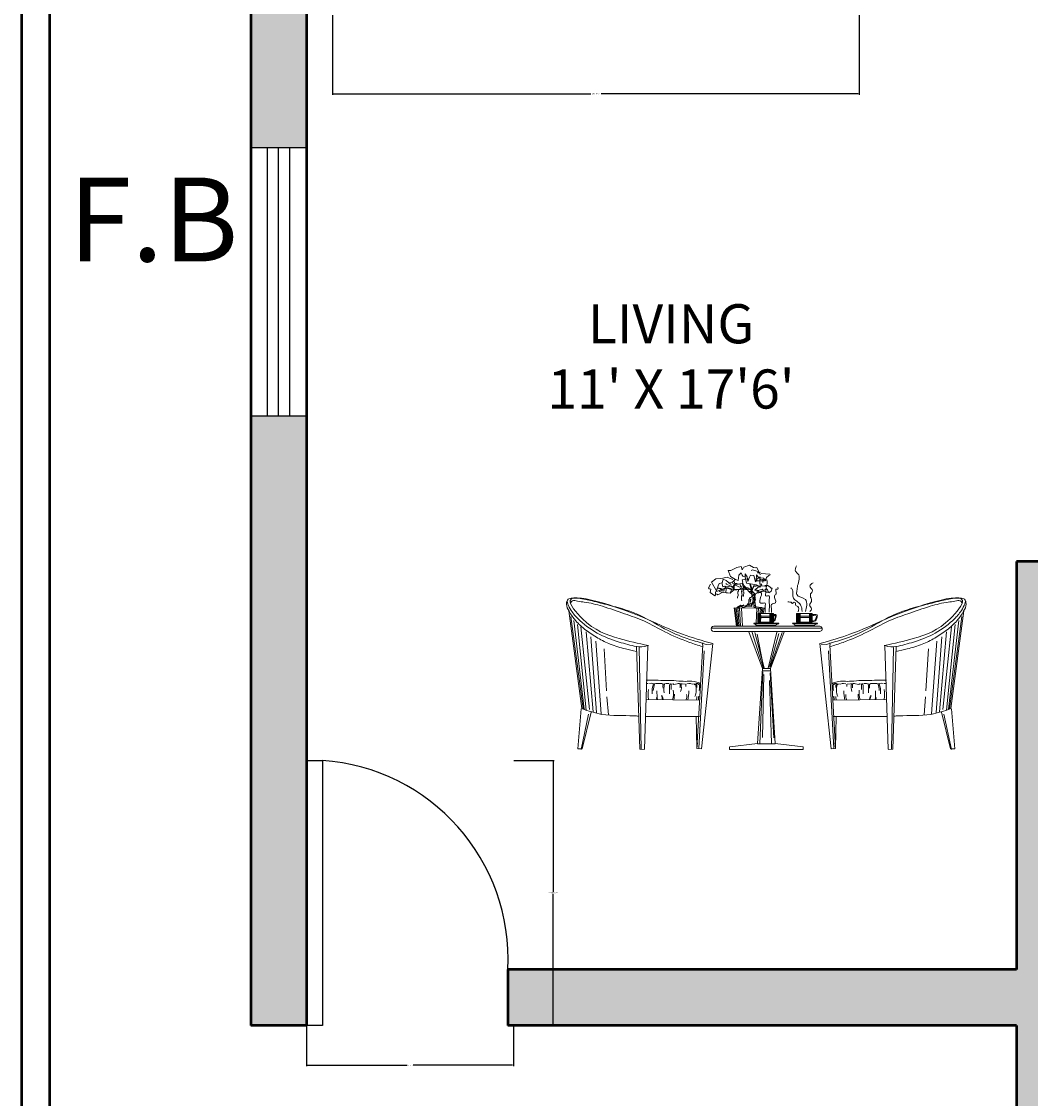
# Model space of a CAD drawing. Units: inches. Extents: x 1771 to 3025, y 319 to 889.
# Tile 26 of 35: x 2683 to 2863, y 521 to 714. Entities that reach past the tile are written whole.
import ezdxf

# ---------------------------------------------------------------- set-up
doc = ezdxf.new("R2010")
doc.units = ezdxf.units.IN
doc.header["$MEASUREMENT"] = 0
for name, color, linetype, lineweight in [('A-ANNO-DIMS', 2, 'Continuous', 18), ('A-AREA-IDEN', 241, 'Continuous', 25), ('A-DOOR', 4, 'Continuous', 25), ('A-FURN', 8, 'Continuous', 18), ('A-GLAZ', 40, 'Continuous', 25), ('A-WALL', 7, 'Continuous', 50), ('A-WALL-PATT', 254, 'Continuous', 13)]:
    doc.layers.add(name, color=color, linetype=linetype, lineweight=lineweight)
doc.styles.get("Standard").update_dxf_attribs({"font": 'arial.ttf'})
doc.dimstyles.get("Standard").update_dxf_attribs({"dimtxt": 0.18, "dimasz": 0.18, "dimexe": 0.18, "dimexo": 0.0625, "dimgap": 0.09, "dimtad": 0, "dimtih": 1, "dimtoh": 1, "dimdec": 4, "dimzin": 0, "dimdsep": 46, "dimtxsty": 'Standard', "dimcen": 0.09, "dimadec": 0, "dimazin": 0, "dimtfac": 1, "dimtdec": 4, "dimtofl": 0, "dimtmove": 0, "dimatfit": 3, "dimfxl": 1, "dimtolj": 1, "dimtzin": 0, "dimarcsym": 0})

# ---------------------------------------------------------------- blocks, each defined once
blk = doc.blocks.new('A$C7D4176DC')
for p, q in [((1010.5, 1037.1), (1041.4, 1048.3)), ((1041.4, 1048.3), (1064.8, 1036.1)), ((914, 980.9), (889.6, 974.3)), ((947.7, 967.8), (914, 980.9)), ((936.5, 1019.3), (919.6, 1018.3)), ((919.6, 1018.3), (933.7, 984.6)), ((933.7, 984.6), (961.8, 966.8)), ((969.3, 1036.1), (936.5, 1019.3)), ((994.5, 1040.8), (969.3, 1036.1)), ((976.7, 961.2), (980.5, 991.2)), ((980.5, 991.2), (994.5, 1005.2)), ((1000.2, 1022.1), (994.5, 1040.8)), ((994.5, 1005.2), (999.2, 992.1)), ((999.2, 992.1), (1006.7, 983.7)), ((1008.6, 1036.1), (1000.2, 1022.1)), ((1006.7, 983.7), (1022.6, 987.4)), ((1022.6, 987.4), (1015.2, 989.3)), ((1029.2, 982.8), (1017, 998.7)), ((1017, 998.7), (1017, 981.8)), ((1017, 981.8), (1024.5, 946.2)), ((1032, 956.5), (1029.2, 982.8)), ((1047.9, 992.1), (1042.3, 979.9)), ((1066.7, 989.3), (1047.9, 992.1)), ((1051.7, 1018.3), (1059.2, 1023)), ((1059.2, 1023), (1090.1, 1013.6)), ((1064.8, 1036.1), (1077, 1034.2)), ((1075.1, 953.7), (1066.7, 989.3)), ((1077, 1034.2), (1084.5, 1035.2)), ((1081.7, 994), (1079.8, 959.4)), ((1095.7, 976.2), (1081.7, 994)), ((1084.5, 1035.2), (1097.6, 1007.1)), ((1103.2, 982.8), (1084.5, 969.7)), ((1091, 1009.9), (1088.2, 1005.2)), ((1088.2, 1005.2), (1104.1, 1009)), ((1090.1, 1013.6), (1091, 1009.9)), ((1104.1, 1009), (1091, 1005.2)), ((1091, 1005.2), (1100.4, 1003.4)), ((1100.4, 1003.4), (1103.2, 993.1)), ((1100.4, 971.5), (1103.2, 982.8)), ((1108.2, 1001.8), (1157.5, 996.8)), ((1151, 989.3), (1137.9, 978.1)), ((1159.4, 994), (1151, 989.3)), ((1157.5, 996.8), (1159.4, 994)), ((820.3, 941.6), (808.1, 920)), ((808.1, 920), (811.9, 913.5)), ((850.3, 971.5), (825.9, 951.9)), ((825.9, 951.9), (853.1, 902.3)), ((879.3, 973.4), (850.3, 971.5)), ((853.1, 902.3), (863.4, 931.3)), ((863.4, 931.3), (869, 944.4)), ((869, 944.4), (886.8, 949.1)), ((889.6, 974.3), (879.3, 973.4)), ((890.6, 924.7), (884, 950)), ((886.8, 949.1), (892.4, 968.7)), ((900.9, 928.5), (890.6, 924.7)), ((892.4, 968.7), (908.4, 962.2)), ((922.4, 927.5), (900.9, 928.5)), ((903.7, 927.5), (902.7, 916.3)), ((905.6, 928.5), (903.7, 927.5)), ((904.6, 923.8), (905.6, 928.5)), ((904.6, 920), (904.6, 923.8)), ((919.6, 920), (904.6, 920)), ((908.4, 962.2), (934.6, 940.6)), ((909.3, 940.6), (908.4, 947.2)), ((917.7, 936), (909.3, 940.6)), ((928, 933.1), (917.7, 936)), ((939.3, 913.5), (919.6, 920)), ((932.7, 929.4), (922.4, 927.5)), ((927.4, 947.9), (955.2, 956.5)), ((942.1, 925.7), (928, 933.1)), ((941.1, 929.4), (932.7, 929.4)), ((934.6, 940.6), (938.3, 938.8)), ((951.5, 911.6), (941.1, 929.4)), ((950.5, 917.2), (942.1, 925.7)), ((946.8, 953.7), (945.8, 946.2)), ((945.8, 946.2), (971.1, 945.3)), ((958, 965.9), (946.8, 953.7)), ((955.2, 940.6), (946.8, 924.7)), ((946.8, 924.7), (951.5, 918.2)), ((959.9, 938.8), (951.5, 925.7)), ((951.5, 925.7), (954.3, 912.5)), ((954.3, 909.7), (955.2, 940.6)), ((955.2, 956.5), (961.8, 934.1)), ((986.1, 943.4), (960.8, 940.6)), ((961.8, 966.8), (976.7, 961.2)), ((961.8, 934.1), (984.2, 923.8)), ((967.4, 939.2), (999.2, 945.3)), ((984.2, 923.8), (995.5, 925.7)), ((989.9, 930.3), (986.1, 943.4)), ((989.5, 915.7), (998.5, 919.9)), ((995.5, 925.7), (989.9, 930.3)), ((998.5, 919.9), (1000.6, 912.2)), ((999.2, 965.9), (1016.1, 967.8)), ((1003, 952.8), (999.2, 965.9)), ((999.2, 945.3), (1003, 952.8)), ((1002, 948.1), (1001.1, 940.6)), ((1001.1, 940.6), (1006.7, 926.6)), ((1012.3, 931.3), (1002, 948.1)), ((1007.7, 920), (1005.8, 917.2)), ((1006.7, 926.6), (1011.4, 921.9)), ((1027.3, 916.3), (1007.7, 920)), ((1009.7, 920.6), (1011.8, 911.5)), ((1011.4, 921.9), (1025.5, 914.4)), ((1021.7, 921.9), (1012.3, 931.3)), ((1016.1, 967.8), (1017, 970.6)), ((1017, 970.6), (1037.6, 969.7)), ((1033, 919.1), (1021.7, 921.9)), ((1024.5, 946.2), (1082.6, 936)), ((1042.3, 979.9), (1032, 956.5)), ((1037.6, 969.7), (1033, 971.5)), ((1047.9, 941.6), (1043.3, 939.7)), ((1043.3, 939.7), (1048.9, 920)), ((1055.4, 914.4), (1047.9, 941.6)), ((1048.9, 920), (1049.8, 910.7)), ((1067.6, 934.1), (1054.5, 910.7)), ((1064.8, 923.8), (1061.1, 918.2)), ((1067.6, 929.4), (1064.8, 927.5)), ((1066.7, 926.6), (1064.8, 923.8)), ((1089.2, 931.3), (1066.7, 926.6)), ((1084.5, 932.2), (1067.6, 929.4)), ((1079.8, 959.4), (1075.1, 953.7)), ((1078.2, 913), (1100.1, 932)), ((1082.6, 936), (1096.7, 928.5)), ((1084.5, 969.7), (1084.5, 959.4)), ((1084.5, 959.4), (1127.6, 960.3)), ((1121, 975.3), (1095.7, 976.2)), ((1096.7, 928.5), (1101.3, 922.8)), ((1100.1, 932), (1097.2, 927.6)), ((1097.2, 927.6), (1117.7, 930.5)), ((1101.3, 940.6), (1100.4, 971.5)), ((1101.3, 922.8), (1111.6, 941.6)), ((1111.6, 941.6), (1101.3, 940.6)), ((1106, 966.8), (1104.1, 968.7)), ((1121, 969.7), (1106, 966.8)), ((1117.7, 930.5), (1139.6, 927.6)), ((1119.1, 963.1), (1121, 969.7)), ((1127.6, 960.3), (1119.1, 963.1)), ((1132.2, 960.3), (1121, 975.3)), ((1129.4, 933.4), (1145.5, 933.4)), ((1137.9, 978.1), (1132.2, 960.3)), ((1145.5, 933.4), (1160.1, 923.2)), ((1160.1, 923.2), (1166, 918.8)), ((811.9, 913.5), (821.2, 911.6)), ((821.2, 911.6), (817.5, 893.8)), ((817.5, 893.8), (843.7, 875.1)), ((843.7, 875.1), (847.5, 880.7)), ((847.5, 897.6), (877.4, 906)), ((847.5, 880.7), (847.5, 897.6)), ((862.1, 880.4), (853.9, 886.5)), ((860.6, 917.2), (858.7, 916.3)), ((863.4, 917.2), (860.6, 917.2)), ((878.4, 916.3), (861.5, 919.1)), ((886.7, 892.7), (862.1, 880.4)), ((876.5, 911.6), (863.4, 917.2)), ((870.3, 898.8), (868.3, 907)), ((895, 892.7), (870.3, 898.8)), ((879.3, 906.9), (876.5, 911.6)), ((877.4, 906), (884.9, 905.1)), ((883.1, 912.5), (878.4, 916.3)), ((894.3, 912.5), (879.3, 906.9)), ((910.2, 917.2), (883.1, 912.5)), ((884.9, 905.1), (889.6, 903.2)), ((889.6, 903.2), (895.2, 901.3)), ((902.7, 916.3), (894.3, 912.5)), ((931.9, 888.6), (895, 892.7)), ((895.2, 901.3), (899, 917.2)), ((909.3, 913.2), (907.3, 892.7)), ((917.5, 890.6), (909.3, 890.6)), ((939.3, 910.7), (910.2, 917.2)), ((931.9, 888.6), (917.5, 890.6)), ((940.1, 909.1), (931.9, 888.6)), ((950.4, 907), (931.9, 888.6)), ((985.2, 912.5), (939.3, 910.7)), ((1026.4, 913.5), (950.4, 907.4)), ((952.4, 910.7), (950.5, 917.2)), ((951.5, 918.2), (951.5, 911.6)), ((954.3, 912.5), (954.3, 909.7)), ((977.6, 875.3), (973.4, 867.6)), ((973.4, 867.6), (973.4, 860.6)), ((976.2, 896.9), (974.8, 892)), ((974.8, 892), (977.6, 877.4)), ((978.3, 903.2), (976.2, 896.9)), ((977.6, 912.2), (978.3, 903.2)), ((977.6, 877.4), (977.6, 875.3)), ((988.9, 914.4), (985.2, 912.5)), ((991.7, 916.3), (988.9, 914.4)), ((1005.8, 917.2), (991.7, 916.3)), ((998.5, 904.6), (995.7, 898.3)), ((995.7, 898.3), (999.9, 878.8)), ((997.1, 872.5), (996.4, 855.8)), ((999.9, 878.8), (997.1, 872.5)), ((1000.6, 912.2), (998.5, 904.6)), ((1006.9, 906), (1004.1, 898.3)), ((1004.1, 898.3), (1009, 894.8)), ((1008.3, 872.5), (1004.8, 871.8)), ((1011.8, 911.5), (1006.9, 906)), ((1006.9, 911.5), (1030.6, 908)), ((1009, 889.2), (1006.9, 877.4)), ((1006.9, 877.4), (1008.3, 872.5)), ((1009, 894.8), (1009, 889.2)), ((1025.5, 914.4), (1048.9, 908.8)), ((1030.6, 908), (1036.9, 901.1)), ((1046.7, 908.7), (1033, 919.1)), ((1036.9, 901.1), (1049.5, 899)), ((1039, 899), (1045.3, 891.3)), ((1049.5, 899), (1039, 899)), ((1044.6, 864.1), (1039.7, 853)), ((1050.9, 864.8), (1044.6, 864.1)), ((1045.3, 891.3), (1052.3, 886.4)), ((1048.9, 908.8), (1076, 881.7)), ((1049.8, 910.7), (1050.8, 902.3)), ((1050.8, 902.3), (1060.1, 872.3)), ((1058.2, 880.7), (1050.8, 894.8)), ((1055.8, 873.9), (1050.9, 864.8)), ((1052.3, 886.4), (1057.9, 876.7)), ((1054.5, 910.7), (1054.5, 898.5)), ((1054.5, 898.5), (1059.9, 896.9)), ((1056.4, 890.1), (1055.4, 914.4)), ((1056.4, 905.1), (1055.4, 895.7)), ((1055.4, 895.7), (1057.3, 892)), ((1057.9, 876.7), (1055.8, 873.9)), ((1061.1, 918.2), (1056.4, 905.1)), ((1064.4, 865.4), (1056.9, 822.4)), ((1060.1, 872.3), (1058.2, 880.7)), ((1069.5, 859.2), (1059.2, 870.4)), ((1065.7, 884.5), (1061.1, 875.1)), ((1061.1, 875.1), (1061.1, 857.3)), ((1064.8, 853.6), (1069.5, 859.2)), ((1074.2, 859.2), (1065.7, 884.5)), ((1070.4, 864.8), (1065.7, 823.6)), ((1070.4, 862.9), (1067.6, 890.1)), ((1076, 851.7), (1070.4, 864.8)), ((1074.2, 829.2), (1070.4, 862.9)), ((1076, 881.7), (1071.4, 876)), ((1071.4, 876), (1073.2, 863.9)), ((1072.3, 910), (1078.2, 913)), ((1091.3, 904.2), (1072.3, 910)), ((1073.2, 863.9), (1074.2, 859.2)), ((1076.7, 886.6), (1073.8, 883.7)), ((1097.2, 895.4), (1076.7, 886.6)), ((1098.6, 893.9), (1089.9, 904.2)), ((1113.3, 911.5), (1091.3, 904.2)), ((1113.3, 902.7), (1097.2, 895.4)), ((1113.3, 899.8), (1098.6, 893.9)), ((1122.1, 904.2), (1113.3, 911.5)), ((1127.9, 901.3), (1113.3, 899.8)), ((1138.2, 914.4), (1122.1, 904.2)), ((1138.2, 895.4), (1127.9, 901.3)), ((1144, 908.6), (1138.2, 914.4)), ((1151.3, 895.4), (1138.2, 895.4)), ((1151.3, 891), (1144, 908.6)), ((1166, 901.3), (1151.3, 891)), ((1166, 918.8), (1170.4, 917.3)), ((1170.4, 917.3), (1166, 901.3)), ((968.4, 700.9), (955.2, 806.2)), ((955.2, 806.2), (1126.5, 803.3)), ((959.3, 806.1), (972.5, 701.9)), ((965.6, 806.1), (976.7, 700.5)), ((991.6, 820.2), (969.9, 808.3)), ((975.3, 805.4), (983, 701.2)), ((979.4, 811.3), (977.9, 801.1)), ((991.8, 816.4), (978.6, 806.2)), ((985.8, 805.4), (990.6, 701.9)), ((1016.7, 816), (991.6, 820.2)), ((1003.5, 807.6), (991.8, 816.4)), ((996.2, 804.1), (1001.1, 701.9)), ((996.4, 855.8), (996.4, 850.9)), ((996.4, 850.9), (997.8, 845.3)), ((1009.4, 822.3), (1002, 816.4)), ((1002, 816.4), (1054.7, 813.5)), ((1013.7, 810.6), (1003.5, 807.6)), ((1041.6, 819.3), (1013.7, 810.6)), ((1060.6, 835.8), (1015.2, 815.4)), ((1022.3, 819.5), (1016.7, 816)), ((1024.4, 819.5), (1022.3, 819.5)), ((1026.5, 819.5), (1024.4, 819.5)), ((1029.9, 828.6), (1026.5, 819.5)), ((1032, 829.3), (1029.9, 828.6)), ((1033.4, 828.6), (1032, 829.3)), ((1036.9, 832), (1033.4, 828.6)), ((1037.6, 834.1), (1036.9, 832)), ((1044.5, 828.1), (1037.2, 822.3)), ((1037.2, 822.3), (1041.6, 819.3)), ((1039, 850.9), (1037.6, 836.2)), ((1037.6, 836.2), (1037.6, 834.1)), ((1039.7, 853), (1039, 850.9)), ((1048.9, 832.5), (1044.5, 828.1)), ((1048.1, 856.4), (1045.3, 850.2)), ((1045.3, 850.2), (1045.3, 839)), ((1045.3, 839), (1048.1, 841.1)), ((1048.1, 841.1), (1048.8, 853.7)), ((1048.8, 853.7), (1048.8, 857.1)), ((1057.7, 829.6), (1048.9, 832.5)), ((1049.8, 817.1), (1076, 851.7)), ((1051.7, 827.4), (1049.8, 817.1)), ((1054.7, 813.5), (1057.7, 829.6)), ((1061.1, 857.3), (1064.8, 853.6)), ((1065.7, 823.6), (1077, 814.3)), ((1066.4, 817.9), (1066.4, 812)), ((1066.4, 812), (1075.2, 806.2)), ((1075.2, 806.2), (1073.8, 812)), ((1073.8, 812), (1114.7, 807.6)), ((1077, 814.3), (1074.2, 829.2)), ((1098.2, 804.7), (1077.7, 804.7)), ((1083.8, 803.4), (1080.4, 718.8)), ((1093.6, 804.7), (1091.9, 774.3)), ((1114.7, 807.6), (1097.2, 801.8)), ((1104, 802), (1101.5, 774.3)), ((1110.9, 799.9), (1108, 774.3)), ((1117.9, 803.4), (1113.7, 774.3)), ((1125, 803.3), (1120, 774.3)), ((13.4, 788.5), (86.9, 232)), ((24.7, 755.7), (94.7, 231.2)), ((976.6, 787.5), (968.6, 786.7)), ((968.6, 786.7), (971.7, 756.8)), ((971.7, 756.8), (979.7, 757.6)), ((979.7, 757.6), (976.6, 787.5)), ((1088.8, 774.3), (1088.8, 724.7)), ((1179, 774.3), (1088.8, 774.3)), ((1100.8, 759), (1088.8, 759)), ((1100.8, 751.4), (1090.1, 751.4)), ((1090.9, 774.1), (1090.9, 725.1)), ((1093.9, 773.8), (1093.9, 725.1)), ((1098.4, 774.1), (1098.4, 724.9)), ((1100.8, 763.6), (1100.8, 747.6)), ((1107.3, 763.6), (1100.8, 763.6)), ((1100.8, 747.6), (1107.3, 747.6)), ((1101.3, 745), (1101.3, 740.5)), ((1107.3, 745), (1101.3, 745)), ((1101.3, 740.5), (1107.3, 740.5)), ((1104.1, 773.8), (1104.1, 763.6)), ((1104.1, 747.6), (1104.1, 745)), ((1104.1, 740.5), (1104.1, 724.7)), ((1107.3, 747.6), (1107.3, 763.6)), ((1179, 759), (1107.3, 759)), ((1179, 751.4), (1107.3, 751.4)), ((1107.3, 740.5), (1107.3, 745)), ((1158.2, 773.8), (1158.2, 725.1)), ((1164.1, 773.8), (1164.1, 724.9)), ((1168.6, 774.3), (1168.6, 725.4)), ((1172.9, 774.1), (1172.9, 767.4)), ((1172.9, 762.7), (1172.9, 734.9)), ((1175.9, 774.1), (1175.9, 767.3)), ((1175.9, 762.6), (1175.9, 734.6)), ((1178, 773.8), (1178, 767.2)), ((1178.3, 762.6), (1178.3, 734.8)), ((1179, 767.3), (1179, 774.3)), ((1179, 734.4), (1179, 762.7)), ((1309.2, 774.3), (1309.2, 724.7)), ((1399.4, 774.3), (1309.2, 774.3)), ((1319.1, 759), (1309.2, 759)), ((1319.1, 751.4), (1310.5, 751.4)), ((1311, 774.3), (1311, 725)), ((1313.8, 774.6), (1313.8, 724)), ((1318.3, 774.3), (1318.3, 725.2)), ((1319.1, 764.9), (1319.1, 742.2)), ((1323.5, 764.9), (1319.1, 764.9)), ((1319.1, 742.2), (1323.5, 742.2)), ((1319.8, 739.2), (1319.8, 735.6)), ((1322.7, 739.2), (1319.8, 739.2)), ((1322.7, 735.6), (1322.7, 739.2)), ((1323.5, 742.2), (1323.5, 764.9)), ((1399.4, 759), (1323.5, 759)), ((1399.4, 751.4), (1323.5, 751.4)), ((1324.3, 774.1), (1324.3, 725.5)), ((1331.2, 774.1), (1331.2, 725)), ((1383.9, 774.1), (1383.9, 725.2)), ((1389.2, 774.1), (1389.2, 724.8)), ((1393.7, 774.1), (1393.7, 724.5)), ((1396.6, 774.1), (1396.6, 724.8)), ((1398.3, 774.1), (1398.3, 724.8)), ((1399.4, 724.7), (1399.4, 774.3)), ((2250.4, 755.7), (2180.4, 231.2)), ((2261.7, 788.5), (2188.2, 232)), ((41.1, 733.1), (100.8, 229.1)), ((61.7, 710.4), (111.1, 223)), ((82.3, 698.1), (131.7, 227.1)), ((1452.4, 690.9), (826.8, 690.9)), ((1438.5, 700.9), (838.5, 700.9)), ((1107.4, 700.9), (968.4, 700.9)), ((1206.9, 718.8), (1068.5, 718.8)), ((1205.1, 715), (1070.7, 715)), ((1079.9, 707.4), (1079.6, 701.2)), ((1192.2, 706.1), (1080.1, 706.6)), ((1191.5, 704.8), (1081.7, 704.8)), ((1083.3, 700.5), (1083.3, 704.5)), ((1088.8, 724.7), (1179, 724.7)), ((1093.2, 718.3), (1093.2, 724.5)), ((1172.9, 732.2), (1172.9, 725.1)), ((1173.3, 725.1), (1173.3, 718.3)), ((1175.9, 731.8), (1175.9, 724.6)), ((1178.3, 731.3), (1178.3, 725.1)), ((1179, 724.7), (1179, 731.4)), ((1189, 704.5), (1189, 700.5)), ((1427.3, 718.8), (1288.9, 718.8)), ((1425.4, 715), (1291, 715)), ((1412.6, 706.1), (1300.5, 706.6)), ((1411.9, 704.8), (1302.1, 704.8)), ((1303.7, 700.5), (1303.7, 704.5)), ((1309.2, 724.7), (1399.4, 724.7)), ((1313.5, 718.3), (1313.5, 724.5)), ((1319.8, 735.6), (1322.7, 735.6)), ((1393.7, 725.1), (1393.7, 718.3)), ((1409.4, 704.5), (1409.4, 700.5)), ((2192.8, 698.1), (2143.4, 227.1)), ((2213.3, 710.4), (2163.9, 223)), ((2233.9, 733.1), (2174.2, 229.1)), ((111.1, 669.3), (152.3, 214.7)), ((137.9, 640.5), (170.8, 210.6)), ((166.7, 615.8), (197.6, 202.4)), ((1438.5, 670.9), (838.5, 670.9)), ((1037.2, 670.1), (1115.4, 459.8)), ((1054.9, 670.7), (1122.1, 460.1)), ((1073, 665.2), (1125.7, 463.7)), ((1085.8, 656.2), (1122.1, 471)), ((1198.4, 667), (1147.5, 461.9)), ((1209.3, 659.8), (1156.6, 467.4)), ((1227.5, 665.2), (1160.2, 467.4)), ((1239.7, 670.1), (1161.5, 459.8)), ((2108.4, 615.8), (2077.5, 202.4)), ((2137.2, 640.5), (2104.3, 210.6)), ((2163.9, 669.3), (2122.8, 214.7)), ((214, 572.6), (228.4, 334)), ((398.7, 587.3), (417.4, 0.9)), ((413.7, 579.8), (424.7, 0.9)), ((462.3, 591), (443.8, 0.9)), ((776.4, 594.8), (742.7, 4.4)), ((783.9, 560.6), (752.8, 5.4)), ((795.6, 597.2), (767.4, 606)), ((832.5, 602.2), (768.9, 2.8)), ((772.6, 598.5), (776.4, 598.5)), ((825, 598.5), (795.6, 597.2)), ((1442.6, 602.2), (1506.2, 2.8)), ((1450.1, 598.5), (1479.4, 597.2)), ((1479.4, 597.2), (1507.7, 606)), ((1491.2, 560.6), (1522.3, 5.4)), ((1502.4, 598.5), (1498.7, 598.5)), ((1498.7, 594.8), (1532.3, 4.4)), ((1812.8, 591), (1831.2, 0.9)), ((1861.4, 579.8), (1850.3, 0.9)), ((1876.4, 587.3), (1857.7, 0.9)), ((2061, 572.6), (2046.6, 334)), ((1115.4, 459.8), (1088.3, 33.1)), ((1118.5, 442), (1100.3, 33.5)), ((1163.9, 447.4), (1114.8, 447.4)), ((1161.5, 459.8), (1115.4, 459.8)), ((1160.2, 436.5), (1180.2, 66.2)), ((1161.5, 459.8), (1188.6, 33.1)), ((465.7, 375.8), (456.5, 375.8)), ((484.1, 377.3), (471.9, 374.3)), ((499.5, 372.7), (484.1, 377.3)), ((508.7, 374.3), (499.5, 372.7)), ((513.3, 375.8), (508.7, 374.3)), ((525.5, 375.8), (513.3, 375.8)), ((531.7, 374.3), (525.5, 375.8)), ((543.9, 374.3), (531.7, 374.3)), ((547, 371.2), (543.9, 374.3)), ((567, 375.8), (547, 371.2)), ((582.3, 374.3), (567, 375.8)), ((593, 371.2), (590, 374.3)), ((606.8, 372.7), (593, 371.2)), ((611.4, 369.7), (606.8, 372.7)), ((629.8, 372.7), (611.4, 369.7)), ((636, 374.3), (629.8, 372.7)), ((643.6, 375.8), (636, 374.3)), ((648.2, 372.7), (643.6, 375.8)), ((659, 372.7), (648.2, 372.7)), ((677.4, 371.2), (659, 372.7)), ((678.9, 371.2), (678.9, 359)), ((697.3, 374.3), (685.1, 372.7)), ((706.5, 374.3), (697.3, 374.3)), ((715.7, 371.2), (706.5, 374.3)), ((729.5, 372.7), (715.7, 371.2)), ((740.3, 374.3), (729.5, 368.2)), ((729.5, 368.2), (729.5, 372.7)), ((747.9, 374.3), (740.3, 374.3)), ((751, 369.7), (747.9, 374.3)), ((760.2, 374.3), (751, 369.7)), ((1123.9, 427.4), (1116.6, 68)), ((1154.8, 393), (1167.5, 35.4)), ((1514.9, 374.3), (1524.1, 369.7)), ((1524.1, 369.7), (1527.1, 374.3)), ((1527.1, 374.3), (1534.8, 374.3)), ((1534.8, 374.3), (1545.5, 368.2)), ((1545.5, 372.7), (1559.3, 371.2)), ((1545.5, 368.2), (1545.5, 372.7)), ((1559.3, 371.2), (1568.5, 374.3)), ((1568.5, 374.3), (1577.7, 374.3)), ((1577.7, 374.3), (1590, 372.7)), ((1596.2, 371.2), (1596.2, 359)), ((1597.7, 371.2), (1616.1, 372.7)), ((1616.1, 372.7), (1626.8, 372.7)), ((1626.8, 372.7), (1631.4, 375.8)), ((1631.4, 375.8), (1639.1, 374.3)), ((1639.1, 374.3), (1645.2, 372.7)), ((1645.2, 372.7), (1663.6, 369.7)), ((1663.6, 369.7), (1668.2, 372.7)), ((1668.2, 372.7), (1682, 371.2)), ((1682, 371.2), (1685.1, 374.3)), ((1692.8, 374.3), (1708.1, 375.8)), ((1708.1, 375.8), (1728.1, 371.2)), ((1728.1, 371.2), (1731.1, 374.3)), ((1731.1, 374.3), (1743.4, 374.3)), ((1743.4, 374.3), (1749.5, 375.8)), ((1749.5, 375.8), (1761.8, 375.8)), ((1761.8, 375.8), (1766.4, 374.3)), ((1766.4, 374.3), (1775.6, 372.7)), ((1775.6, 372.7), (1790.9, 377.3)), ((1790.9, 377.3), (1803.2, 374.3)), ((1809.3, 375.8), (1818.5, 375.8)), ((230.5, 299.1), (238.7, 196.2)), ((756.8, 280.8), (451.1, 284.6)), ((1518.3, 280.8), (1824, 284.6)), ((2044.6, 299.1), (2036.3, 196.2)), ((84, 230.1), (64.2, 2.8)), ((126, 200.5), (84, 0.3)), ((140.9, 212.8), (88.9, 2.8)), ((447.3, 187.5), (757.7, 187.5)), ((739, 187.5), (742.7, 4.4)), ((1827.8, 187.5), (1517.4, 187.5)), ((1536.1, 187.5), (1532.3, 4.4)), ((2134.2, 212.8), (2186.2, 2.8)), ((2149.1, 200.5), (2191.1, 0.3)), ((2191.1, 230.1), (2210.9, 2.8)), ((64.2, 2.8), (88.9, 2.8)), ((417.4, 0.9), (443.8, 0)), ((742.7, 4.4), (746.5, 38)), ((742.7, 4.4), (768.9, 2.8)), ((927.1, 15), (927.1, 0)), ((1088.3, 33.1), (929, 15)), ((1187.5, 31.7), (1087.6, 31.7)), ((1188.6, 33.1), (1348, 15)), ((1348, 15), (1348, 0)), ((1532.3, 4.4), (1506.2, 2.8)), ((1532.3, 4.4), (1528.6, 38)), ((1857.7, 0.9), (1831.3, 0)), ((2210.9, 2.8), (2186.2, 2.8)), ((1348, 0), (927.1, 0))]:
    blk.add_line(p, q)
for centre, radius, start, end in [((838.2, 685.9), 15, 89.02539, 270.97461), ((1069.4, 716.9), 2.21, 114.75071, 294.8305), ((1059.6, 691.4), 25.9, 31.12717, 65.45392), ((1208.6, 696.5), 19, 99.79621, 154.31096), ((1206.2, 716.7), 1.95, 244.55032, 96.50843), ((1289.8, 716.9), 2.21, 114.75071, 294.8305), ((1280, 691.4), 25.9, 31.12717, 65.45392), ((1429, 696.5), 19, 99.79621, 154.31096), ((1426.6, 716.7), 1.95, 244.55032, 96.50843), ((1440.2, 685.9), 15.1, 263.50595, 96.49405), ((421.9, 675.7), 92.7, 253.90068, 295.36386), ((1853.1, 675.7), 92.7, 244.63614, 286.09932), ((631.7, 325.3), 145, 160.46362, 183.26427), ((661.3, 321.8), 167.8, 162.1481, 175.52768), ((592, 359.5), 42.9, 161.29008, 193.50095), ((755.4, 341.1), 200.6, 170.95256, 185.34949), ((841.5, 337.8), 255.8, 172.03905, 184.65389), ((943.9, 345.9), 348.8, 175.42446, 180.75439), ((590.6, 356.2), 56.7, 354.25823, 16.89433), ((579.3, 354.7), 74.8, 340.32989, 13.94105), ((619.9, 341.7), 118.4, 339.52102, 14.35705), ((693.6, 357.6), 48.4, 353.58471, 16.22063), ((689.2, 351.2), 68.2, 347.09902, 16.48344), ((1585.8, 351.2), 68.2, 163.51656, 192.90098), ((1581.5, 357.6), 48.4, 163.77937, 186.41529), ((1655.1, 341.7), 118.4, 165.64295, 200.47898), ((1695.8, 354.7), 74.8, 166.05895, 199.67011), ((1684.4, 356.2), 56.7, 163.10567, 185.74177), ((1331.2, 345.9), 348.8, 359.24561, 4.57554), ((1433.6, 337.8), 255.8, 355.34611, 7.96095), ((1519.7, 341.1), 200.6, 354.65051, 9.04744), ((1683.1, 359.5), 42.9, 346.49905, 18.70992), ((1613.7, 321.8), 167.8, 4.47232, 17.8519), ((1643.3, 325.3), 145, 356.73573, 19.53638), ((665.2, 310.8), 200.4, 171.53233, 187.34342), ((746.2, 323.3), 231.2, 177.65923, 189.89094), ((596.6, 305.3), 53.4, 177.23164, 203.39317), ((484.6, 319.5), 124.8, 342.71731, 8.30681), ((204.5, 341.5), 411.6, 351.83053, 356.14259), ((645.6, 301.5), 39.5, 333.88539, 14.90767), ((494.8, 326.9), 201, 346.57929, 1.64099), ((1780.3, 326.9), 201, 178.35901, 193.42071), ((1629.4, 301.5), 39.5, 165.09233, 206.11461), ((2070.6, 341.5), 411.6, 183.85741, 188.16947), ((1790.4, 319.5), 124.8, 171.69319, 197.28269), ((1678.5, 305.3), 53.4, 336.60683, 2.76836), ((1528.9, 323.3), 231.2, 350.10906, 2.34077), ((1609.9, 310.8), 200.4, 352.65658, 8.46767), ((522.1, 292), 10.6, 155.04372, 216.38582), ((-475.8, 101.1), 1042.4, 10.14258, 11.10952), ((682.4, 301.4), 59.8, 341.0378, 359.49279), ((616.9, 303.9), 135.6, 349.74606, 359.61704), ((1658.2, 303.9), 135.6, 180.38296, 190.25394), ((1592.7, 301.4), 59.8, 180.50721, 198.9622), ((2750.9, 101.1), 1042.4, 168.89048, 169.85742), ((1753, 292), 10.6, 323.61418, 24.95628)]:
    blk.add_arc(centre, radius, start, end)
for points, knots in [([(1361.4, 785.9), (1364, 797.1), (1369.1, 819), (1366.1, 867.4), (1305.9, 865.7), (1312.3, 906.5), (1315.7, 942.7), (1336.1, 991.6), (1296, 1015.4), (1304.6, 1034), (1310, 1045.7)], [0, 0, 0, 0, 35.255511, 69.327341, 124.802742, 145.944632, 176.486081, 244.459642, 263.687549, 295.971636, 295.971636, 295.971636, 295.971636]), ([(1154.2, 782.2), (1154.8, 800.5), (1155.7, 825.5), (1152.5, 852.8), (1161, 880.4), (1126, 866.1), (1137.2, 896.5), (1131.8, 923.4), (1156.8, 968.1), (1113.4, 971.1), (1116.9, 957), (1118.7, 949.8)], [0, 0, 0, 0, 53.324624, 72.369114, 91.413604, 110.471764, 134.594802, 149.830446, 204.42477, 220.941926, 238.716972, 238.716972, 238.716972, 238.716972]), ([(1166.9, 779.6), (1167.6, 787.2), (1168.9, 801.7), (1159.5, 831.3), (1208.7, 829.6), (1171.7, 871.4), (1202, 885.9), (1182.6, 918), (1207, 909.8), (1204.8, 918.7), (1203.8, 923.1)], [0, 0, 0, 0, 24.123038, 45.706674, 71.213394, 110.655389, 125.899008, 152.561192, 162.725628, 172.882723, 172.882723, 172.882723, 172.882723]), ([(1341.7, 785.9), (1340.2, 798.9), (1337.5, 822.1), (1313, 843.2), (1292.5, 855.8), (1286.2, 880.3), (1292.2, 903.3), (1280.3, 916.5), (1276.7, 920.3)], [0, 0, 0, 0, 37.360481, 67.270583, 93.998428, 104.993238, 141.362472, 156.467713, 156.467713, 156.467713, 156.467713]), ([(1385.6, 784.4), (1390.4, 789.9), (1401.4, 802.3), (1375.2, 822.1), (1401.7, 842.3), (1389.4, 864.6), (1386.5, 887), (1411.5, 904.8), (1373.5, 930.7), (1394.6, 942.4), (1403.7, 947.5)], [0, 0, 0, 0, 18.925439, 42.566292, 64.867201, 90.936936, 109.058775, 128.752565, 161.181972, 185.77482, 185.77482, 185.77482, 185.77482]), ([(398, 584.9), (364.8, 593.1), (288.2, 612.1), (173, 656.7), (78.3, 727.2), (27.8, 785.3), (-11.1, 856.8), (24.4, 860.7), (34.5, 861.8)], [0, 0, 0, 0, 102.450812, 236.341037, 372.740804, 434.264952, 500.538568, 526.867635, 526.867635, 526.867635, 526.867635]), ([(832.5, 602.2), (773.3, 619.4), (552.4, 683.6), (381.9, 796.6), (-38, 894.8), (125.3, 689.4), (274.3, 633.7), (409.7, 603.5), (466, 591)], [0, 0, 0, 0, 179.241333, 669.878405, 853.517726, 978.360591, 1217.111989, 1387.04363, 1387.04363, 1387.04363, 1387.04363]), ([(778, 604.3), (747.1, 612.4), (671.2, 632.3), (544.7, 691), (406.7, 777.8), (262.4, 816.3), (152.4, 843.8), (83.7, 860.5), (45.9, 861.5), (34.5, 861.8)], [0, 0, 0, 0, 95.639299, 234.867324, 416.660896, 581.537135, 678.863317, 758.06805, 792.133261, 792.133261, 792.133261, 792.133261]), ([(1131.4, 779.6), (1130.3, 791.6), (1128.8, 807.5), (1135.2, 839.3), (1091.9, 821.5), (1105.3, 863.2), (1115.5, 900.9), (1079.7, 883.7), (1089.8, 909.5), (1078.6, 906.7), (1072.9, 905.3)], [0, 0, 0, 0, 39.358681, 52.054923, 76.195091, 115.553772, 137.137409, 158.736993, 171.43349, 184.13893, 184.13893, 184.13893, 184.13893]), ([(1442.6, 602.2), (1501.7, 619.4), (1722.7, 683.6), (1893.2, 796.6), (2313.1, 894.8), (2149.7, 689.4), (2000.7, 633.7), (1865.4, 603.5), (1809.1, 591)], [0, 0, 0, 0, 179.241333, 669.878405, 853.517726, 978.360591, 1217.111989, 1387.04363, 1387.04363, 1387.04363, 1387.04363]), ([(1497.1, 604.3), (1528, 612.4), (1603.8, 632.3), (1730.4, 691), (1868.3, 777.8), (2012.7, 816.3), (2122.7, 843.8), (2191.4, 860.5), (2229.2, 861.5), (2240.6, 861.8)], [0, 0, 0, 0, 95.639299, 234.867324, 416.660896, 581.537135, 678.863317, 758.06805, 792.133261, 792.133261, 792.133261, 792.133261]), ([(1877.1, 584.9), (1910.3, 593.1), (1986.9, 612.1), (2102.1, 656.7), (2196.8, 727.2), (2247.3, 785.3), (2286.2, 856.8), (2250.7, 860.7), (2240.6, 861.8)], [0, 0, 0, 0, 102.450812, 236.341037, 372.740804, 434.264952, 500.538568, 526.867635, 526.867635, 526.867635, 526.867635]), ([(397.9, 557.5), (377.2, 562.2), (327.1, 573.6), (252, 594.7), (177.4, 633.5), (110.3, 676.9), (52.9, 727.5), (17.7, 778.4), (-3, 818.5), (1.2, 838.8), (2.4, 844.5)], [0, 0, 0, 0, 63.757158, 154.207673, 233.111021, 314.773872, 393.990027, 459.45949, 503.309158, 520.507412, 520.507412, 520.507412, 520.507412]), ([(774.4, 584.9), (749.6, 592.8), (676.5, 616.3), (565.4, 663.8), (449, 732.3), (326.3, 773), (214.5, 813.5), (122.5, 837.9), (67.5, 840.8), (36.8, 851.9), (27.3, 839.8), (24.3, 836)], [0, 0, 0, 0, 78.234212, 230.212389, 361.399227, 482.184421, 615.817971, 721.353317, 759.79292, 789.08251, 802.845503, 802.845503, 802.845503, 802.845503]), ([(1319.1, 782.9), (1321.9, 795.4), (1325.6, 812.1), (1309.5, 816.4), (1302.3, 822.2), (1305.8, 830.8), (1295.5, 845.6), (1286, 822.9), (1281.2, 839.2), (1270.5, 838.4), (1264.1, 839.6), (1260.1, 840.3)], [0, 0, 0, 0, 30.24085, 40.376736, 46.786017, 54.336911, 66.135106, 80.063877, 89.736225, 97.441532, 109.625491, 109.625491, 109.625491, 109.625491]), ([(1500.6, 584.9), (1525.5, 592.8), (1598.5, 616.3), (1709.7, 663.8), (1826.1, 732.3), (1948.7, 773), (2060.6, 813.5), (2152.5, 837.9), (2207.6, 840.8), (2238.3, 851.9), (2247.7, 839.8), (2250.7, 836)], [0, 0, 0, 0, 78.234212, 230.212389, 361.399227, 482.184421, 615.817971, 721.353317, 759.79292, 789.08251, 802.845503, 802.845503, 802.845503, 802.845503]), ([(1877.1, 557.5), (1897.9, 562.2), (1947.9, 573.6), (2023.1, 594.7), (2097.7, 633.5), (2164.7, 676.9), (2222.2, 727.5), (2257.3, 778.4), (2278.1, 818.5), (2273.8, 838.8), (2272.7, 844.5)], [0, 0, 0, 0, 63.757158, 154.207673, 233.111021, 314.773872, 393.990027, 459.45949, 503.309158, 520.507412, 520.507412, 520.507412, 520.507412]), ([(1169.5, 767.6), (1169.1, 766.9), (1168.6, 765.8), (1168.5, 764.1), (1168.9, 763.4), (1169.1, 763)], [0, 0, 0, 0, 2.454471, 3.694729, 4.863756, 4.863756, 4.863756, 4.863756]), ([(1169.1, 763), (1172.8, 762.7), (1177.7, 762.3), (1183.6, 763.4), (1189.9, 762.9), (1187.4, 754.3), (1187.2, 747.1), (1184.4, 741.1), (1183.6, 734.2), (1179.1, 734.3), (1176.3, 734.5), (1173.7, 734.9), (1171.6, 734.9), (1169.1, 736.3), (1168.8, 734.4), (1168.7, 733.5), (1168.7, 732.9), (1169, 732.2), (1169.6, 732.2), (1169.9, 732.3)], [0, 0, 0, 0, 11.017731, 14.368752, 18.607743, 26.502791, 33.640107, 41.65747, 47.330925, 50.070533, 53.653147, 56.161165, 57.765785, 60.50412, 61.601302, 62.440841, 63.254964, 63.604793, 64.589255, 64.589255, 64.589255, 64.589255]), ([(1169.5, 767.6), (1173.2, 767.4), (1179.9, 766.9), (1197.8, 769.9), (1190.9, 747.3), (1187.7, 728.5), (1175.3, 732.4), (1169.7, 732.3), (1169.1, 732.2)], [0, 0, 0, 0, 11.640419, 20.980802, 45.0396, 57.043585, 71.929427, 73.92866, 73.92866, 73.92866, 73.92866]), ([(1180.5, 766.4), (1182.7, 766.7), (1186, 767.2), (1193.4, 764.4), (1189.7, 753.8), (1188.7, 747.3), (1188.2, 744.3)], [0, 0, 0, 0, 6.446326, 10.075492, 21.292554, 31.027811, 31.027811, 31.027811, 31.027811]), ([(1399.4, 767.3), (1402.9, 767.5), (1411.4, 768.1), (1432.6, 770.2), (1424.9, 746.9), (1419.3, 731), (1409, 728.9), (1399.9, 726.6), (1399.4, 728.7), (1399.4, 728.8)], [0, 0, 0, 0, 11.082717, 27.168464, 47.8303, 63.341794, 75.5235, 81.952599, 82.221535, 82.221535, 82.221535, 82.221535]), ([(1399.4, 760.8), (1402.3, 761.2), (1409.4, 762.1), (1423.2, 766.3), (1423.3, 753.9), (1420.3, 746.4), (1417.8, 735.7), (1409.3, 733.5), (1403.3, 729.7), (1400.4, 731.6), (1399.4, 732.3)], [0, 0, 0, 0, 9.652474, 22.996839, 29.518582, 40.146055, 49.702279, 58.739504, 65.130432, 68.539734, 68.539734, 68.539734, 68.539734]), ([(763.3, 374.3), (771.1, 374), (721.2, 391.5), (701, 387.4), (647.2, 387.1), (600.7, 394.2), (547.4, 391.8), (499.5, 394.7), (467.3, 394.3), (453.5, 394.2)], [0, 0, 0, 0, 23.359127, 69.600901, 112.546095, 167.952511, 215.499051, 270.735631, 312.147322, 312.147322, 312.147322, 312.147322]), ([(1511.8, 374.3), (1504, 374), (1553.9, 391.5), (1574.1, 387.4), (1627.8, 387.1), (1674.4, 394.2), (1727.7, 391.8), (1775.6, 394.7), (1807.8, 394.3), (1821.6, 394.2)], [0, 0, 0, 0, 23.359127, 69.600901, 112.546095, 167.952511, 215.499051, 270.735631, 312.147322, 312.147322, 312.147322, 312.147322]), ([(86.9, 232), (124.5, 219.1), (220.3, 186.2), (332, 194.5), (402.2, 190.3), (411.4, 189.7)], [0, 0, 0, 0, 118.259021, 301.591906, 329.266035, 329.266035, 329.266035, 329.266035]), ([(2188.2, 232), (2150.6, 219.1), (2054.8, 186.2), (1943.1, 194.5), (1872.9, 190.3), (1863.7, 189.7)], [0, 0, 0, 0, 118.259021, 301.591906, 329.266035, 329.266035, 329.266035, 329.266035])]:
    blk.add_open_spline(points, degree=3, knots=knots)
blk = doc.blocks.new('DOOR-36A')
blk.add_lwpolyline([(0, 47.37), (2.84, 47.37), (2.84, 0), (0, 0)], close=True)
blk.add_arc((0.47, 11.87), 35.58, 356.991, 86.1899)
blk = doc.blocks.new('WIN-48')
for p, q in [((0, 0), (0, 10)), ((48, 0), (48, 10)), ((0, 7), (48, 7)), ((0, 5), (48, 5)), ((0, 3), (48, 3))]:
    blk.add_line(p, q)
blk = doc.blocks.new('*D32')
at = {"layer": 'A-ANNO-DIMS', "color": 0, "lineweight": -2, "transparency": 16777216}
for p, q in [((2770.77, 581.85), (2777.99, 581.85)), ((2777.81, 581.67), (2777.81, 558.35)), ((2777.81, 534.66), (2777.81, 557.98)), ((2770.77, 534.48), (2777.99, 534.48))]:
    blk.add_line(p, q, dxfattribs=at)
at = {"layer": 'A-ANNO-DIMS', "color": 0, "transparency": 16777216}
for points in [[(2777.78, 581.67), (2777.84, 581.67), (2777.81, 581.85)], [(2777.78, 534.66), (2777.84, 534.66), (2777.81, 534.48)]]:
    blk.add_solid(points, dxfattribs=at)
at = {"layer": 'Defpoints', "color": 0, "transparency": 16777216}
for p in [(2770.71, 581.85), (2777.81, 581.85), (2770.71, 534.48)]:
    blk.add_point(p, dxfattribs=at)
at = {"layer": 'A-ANNO-DIMS', "color": 0, "transparency": 16777216, "insert": (2777.81, 558.17), "char_height": 0.18, "attachment_point": 5}
blk.add_mtext('\\A1;DOOR D3 47 TYP.', dxfattribs=at)
blk = doc.blocks.new('*D33')
at = {"layer": 'A-ANNO-DIMS', "color": 0, "lineweight": -2, "transparency": 16777216}
for p, q in [((2733.68, 534.42), (2733.68, 527.2)), ((2770.71, 534.42), (2770.71, 527.2)), ((2733.86, 527.38), (2751.67, 527.38)), ((2770.53, 527.38), (2752.72, 527.38))]:
    blk.add_line(p, q, dxfattribs=at)
at = {"layer": 'A-ANNO-DIMS', "color": 0, "transparency": 16777216}
for points in [[(2733.86, 527.41), (2733.86, 527.35), (2733.68, 527.38)], [(2770.53, 527.41), (2770.53, 527.35), (2770.71, 527.38)]]:
    blk.add_solid(points, dxfattribs=at)
at = {"layer": 'Defpoints', "color": 0, "transparency": 16777216}
for p in [(2733.68, 534.48), (2770.71, 534.48), (2770.71, 527.38)]:
    blk.add_point(p, dxfattribs=at)
at = {"layer": 'A-ANNO-DIMS', "color": 0, "transparency": 16777216, "insert": (2752.2, 527.38), "char_height": 0.18, "attachment_point": 5}
blk.add_mtext('\\A1;37 TYP.', dxfattribs=at)
blk = doc.blocks.new('*D46')
at = {"layer": 'A-ANNO-DIMS', "color": 0, "lineweight": -2, "transparency": 16777216}
for p, q in [((2738.34, 715.17), (2738.34, 700.92)), ((2832.56, 715.17), (2832.56, 700.92)), ((2738.52, 701.1), (2784.55, 701.1)), ((2832.38, 701.1), (2786.36, 701.1))]:
    blk.add_line(p, q, dxfattribs=at)
at = {"layer": 'A-ANNO-DIMS', "color": 0, "transparency": 16777216}
for points in [[(2738.52, 701.13), (2738.52, 701.07), (2738.34, 701.1)], [(2832.38, 701.13), (2832.38, 701.07), (2832.56, 701.1)]]:
    blk.add_solid(points, dxfattribs=at)
at = {"layer": 'Defpoints', "color": 0, "transparency": 16777216}
for p in [(2738.34, 715.24), (2832.56, 715.24), (2832.56, 701.1)]:
    blk.add_point(p, dxfattribs=at)
at = {"layer": 'A-ANNO-DIMS', "color": 0, "transparency": 16777216, "insert": (2785.45, 701.1), "char_height": 0.18, "attachment_point": 5}
blk.add_mtext('\\A1;SOFA 94 TYP.', dxfattribs=at)

msp = doc.modelspace()

# ---------------------------------------------------------------- hatches: boundary and pattern name
at = {"layer": 'A-WALL-PATT'}
h = msp.add_hatch(color=256, dxfattribs=at)
h.dxf.hatch_style = 1
h.paths.add_polyline_path([(2870.68, 879.48), (2892.73, 879.48), (2892.73, 889.48), (2842.68, 889.48), (2842.68, 879.48), (2865.68, 879.48), (2865.68, 831.48), (2870.68, 831.48)])
h.paths.add_polyline_path([(2983.64, 889.48), (2940.73, 889.48), (2940.73, 879.48), (2961.68, 879.48), (2961.68, 795.48), (2865.68, 795.48), (2865.68, 759.48), (2865.68, 665.48), (2870.68, 665.48), (2870.68, 712.85), (2870.68, 790.48), (2978.68, 790.48), (2978.68, 795.48), (2966.68, 795.48), (2966.68, 879.48), (2983.64, 879.48)])
h.paths.add_polyline_path([(3024.68, 889.48), (3001.64, 889.48), (3001.64, 879.48), (3014.68, 879.48), (3014.68, 790.48), (3014.68, 769.46), (3024.68, 769.46)])
h.paths.add_polyline_path([(3024.68, 721.46), (3014.68, 721.46), (3014.68, 670.48), (2906.68, 670.48), (2906.68, 665.48), (2925.68, 665.48), (2925.68, 653.48), (2930.68, 653.48), (2930.68, 665.48), (3014.68, 665.48), (3014.68, 650.02), (3024.68, 650.02)])
h.paths.add_polyline_path([(3024.68, 632.02), (3014.68, 632.02), (3014.68, 617.48), (2925.68, 617.48), (2906.68, 617.48), (2906.68, 612.48), (3014.68, 612.48), (3014.68, 581.96), (3024.68, 581.96)])
h.paths.add_polyline_path([(3024.68, 533.96), (3014.68, 533.96), (3014.68, 480.48), (2870.68, 480.48), (2870.68, 617.48), (2860.68, 617.48), (2860.68, 544.48), (2769.68, 544.48), (2769.68, 534.48), (2860.68, 534.48), (2860.68, 470.48), (3014.68, 470.48), (3014.68, 453.61), (3024.68, 453.61)])
h.paths.add_polyline_path([(3024.68, 405.61), (3014.68, 405.61), (3014.68, 394.48), (2860.68, 394.48), (2860.68, 384.48), (3024.68, 384.48)])
h.paths.add_polyline_path([(2733.68, 643.43), (2723.68, 643.43), (2723.68, 534.48), (2733.68, 534.48)])
h.paths.add_polyline_path([(2733.68, 754.48), (2829.68, 754.48), (2829.68, 759.48), (2733.68, 759.48), (2733.68, 843.44, -0.008336), (2732.38, 843.48), (2723.68, 843.48), (2723.68, 691.43), (2733.68, 691.43)])
h.paths.add_polyline_path([(2794.68, 889.48), (2723.68, 889.48), (2723.68, 879.48), (2794.68, 879.48)])

# ---------------------------------------------------------------- linework, layer by layer
at = {"layer": 'A-WALL'}
for p, q in [((2682.68, 889.48), (2682.68, 534.48)), ((2687.68, 879.48), (2687.68, 534.48)), ((2723.68, 843.48), (2723.68, 534.48)), ((2733.68, 754.48), (2733.68, 534.48)), ((2870.68, 617.48), (2860.68, 617.48)), ((2860.68, 617.48), (2860.68, 544.48)), ((2860.68, 544.48), (2769.68, 544.48)), ((2769.68, 544.48), (2769.68, 534.48)), ((2733.68, 534.48), (2723.68, 534.48)), ((2860.68, 534.48), (2769.68, 534.48)), ((2860.68, 534.48), (2860.68, 470.48))]:
    msp.add_line(p, q, dxfattribs=at)
for points in [[(2682.68, 534.48), (2682.68, 394.48, 0.414214), (2692.68, 384.48), (2860.68, 384.48)], [(2687.68, 534.48), (2687.68, 394.48, 0.414214), (2692.68, 389.48), (2860.68, 389.48)]]:
    msp.add_lwpolyline(points, format="xyb", dxfattribs=at)

# ---------------------------------------------------------------- block references
at = {"layer": 'A-DOOR'}
msp.add_blockref('DOOR-36A', (2733.68, 534.48), dxfattribs=at)
at = {"layer": 'A-FURN', "xscale": 0.0314240770509951, "yscale": 0.0314240770509951, "zscale": 0.0314240770509951}
msp.add_blockref('A$C7D4176DC', (2780.18, 583.84), dxfattribs=at)
at = {"layer": 'A-GLAZ', "rotation": 89.99999999999969}
msp.add_blockref('WIN-48', (2733.68, 643.43), dxfattribs=at)

# ---------------------------------------------------------------- texts
at = {"layer": 'A-AREA-IDEN', "attachment_point": 1}
for s, insert, char_height in [('\\pxqc;F.B', (2663.54, 686.13), 15), ("\\pxqc;LIVING \\P11' X 17'6'", (2756.15, 663.48), 7)]:
    msp.add_mtext_dynamic_manual_height_columns(s, width=85.4611, gutter_width=1, heights=[0], dxfattribs=dict(at, insert=insert, char_height=char_height))

# ---------------------------------------------------------------- dimensions: what is measured, and where the dimension line sits
at = {"layer": 'A-ANNO-DIMS'}
for base, p1, p2, text, picture, middle in [((2832.56, 701.1), (2738.34, 715.24), (2832.56, 715.24), 'SOFA <> TYP.', '*D46', (2785.45, 701.1)), ((2770.71, 527.38), (2733.68, 534.48), (2770.71, 534.48), '<> TYP.', '*D33', (2752.2, 527.38))]:
    dim = msp.add_linear_dim(base=base, p1=p1, p2=p2, text=text, dimstyle='Standard', override={"dimdec": 0, "dimrnd": 0, "dimzin": 0, "dimlunit": 2}, dxfattribs=at)
    dim.commit()
    dim.dimension.update_dxf_attribs({"geometry": picture, "text_midpoint": middle})
dim = msp.add_linear_dim(base=(2777.81, 581.85), p1=(2770.71, 534.48), p2=(2770.71, 581.85), angle=90, text='DOOR D3 <> TYP.', dimstyle='Standard', override={"dimdec": 0, "dimrnd": 0, "dimzin": 0, "dimlunit": 2}, dxfattribs=at)
dim.commit()
dim.dimension.update_dxf_attribs({"geometry": '*D32', "text_midpoint": (2777.81, 558.17)})

doc.saveas('drawing.dxf')
